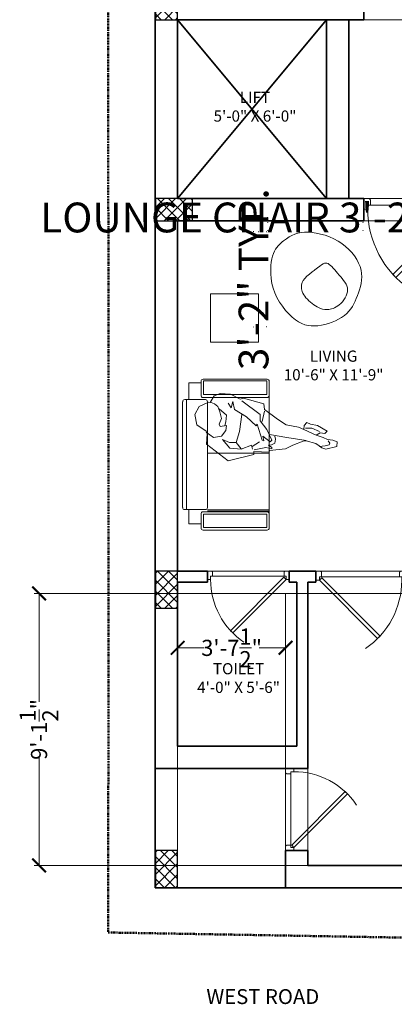
# Model space of a CAD drawing. Units: inches. Extents: x -16911 to -9621, y -48626 to -46270.
# Tile 11 of 20: x -12116 to -11965, y -46992 to -46595. Entities that reach past the tile are written whole.
import ezdxf

# ---------------------------------------------------------------- set-up
doc = ezdxf.new("R2010")
doc.units = ezdxf.units.IN
for name, pattern in [('DASHDOT', [1, 0.5, -0.25, 0, -0.25]), ('DASHED', [19.05, 12.7, -6.35]), ('DOT2', [3.175, 0, -3.175])]:
    doc.linetypes.add(name, pattern=pattern)
for name, color, linetype, lineweight in [('A-ANNO-DIMS', 2, 'Continuous', 13), ('A-ANNO-TEXT', 7, 'Continuous', 18), ('A-AREA-IDEN', 3, 'Continuous', 18), ('A-DOOR', 4, 'Continuous', 18), ('A-FURN', 8, 'Continuous', 13), ('A-WALL', 7, 'Continuous', 35), ('C-PROP', 6, 'DASHDOT', 50), ('column', 12, 'Continuous', 30), ('DOOR', 143, 'Continuous', 9), ('EXT BEAM', 132, 'Continuous', 13), ('furniture', 35, 'Continuous', 15), ('Man', 8, 'Continuous', 5), ('S-BEAM', 132, 'Continuous', 25), ('S-COLS', 1, 'Continuous', 30)]:
    doc.layers.add(name, color=color, linetype=linetype, lineweight=lineweight)
doc.styles.add('style3', font='times.ttf')
doc.styles.add('style9', font='swisscl.ttf', dxfattribs={"height": 12})
doc.dimstyles.new('Dim9', dxfattribs={"dimtxt": 10, "dimasz": 0.199219, "dimexe": 1, "dimexo": 0.5, "dimgap": 1, "dimtad": 0, "dimdec": 1, "dimzin": 0, "dimdsep": 46, "dimlunit": 4, "dimtxsty": 'style9', "dimblk": 'ARCHTICK', "dimcen": 0.09, "dimclrd": 256, "dimclrt": 256, "dimadec": 0, "dimazin": 0, "dimtfac": 1, "dimtdec": 1, "dimtix": 1, "dimtofl": 0, "dimtmove": 1, "dimatfit": 3, "dimfxl": 9, "dimtolj": 1, "dimtzin": 0, "dimlwd": -1, "dimarcsym": 0})
doc.dimstyles.new('S.S.S', dxfattribs={"dimtxt": 6.5, "dimasz": 5.5, "dimexe": 2, "dimexo": 0, "dimgap": 0.09, "dimtad": 0, "dimdec": 1, "dimzin": 3, "dimdsep": 46, "dimlunit": 4, "dimtxsty": 'style3', "dimblk": 'ARCHTICK', "dimcen": 2.5, "dimclrd": 252, "dimclre": 256, "dimclrt": 7, "dimadec": 0, "dimazin": 0, "dimtfac": 1, "dimtdec": 1, "dimtix": 1, "dimtofl": 0, "dimtmove": 0, "dimatfit": 3, "dimfxl": 2, "dimtolj": 1, "dimtzin": 0, "dimlwd": 13, "dimlwe": 15, "dimarcsym": 0})

# ---------------------------------------------------------------- blocks, each defined once
blk = doc.blocks.new('Bipman02')
blk.add_lwpolyline([(0.5871, -0.067), (0.6175, -0.0496), (0.6523, -0.0539), (0.6697, -0.0376), (0.5958, 0.0069), (0.5437, 0.0156), (0.5164, 0.0297), (0.4959, 0.0069), (0.4915, -0.0235), (0.4524, -0.0061), (0.3568, 0.0113), (0.2917, 0.0548), (0.1917, 0.1287), (0.1874, 0.1722), (0.031, 0.2156), (0.0049, 0.2069), (-0.0689, 0.2461), (-0.1471, 0.2504), (-0.1949, 0.233), (-0.2253, 0.1808), (-0.2384, 0.1852), (-0.3079, 0.1504), (-0.3426, 0.0895), (-0.3253, 0.0113), (-0.2558, -0.0365), (-0.2471, -0.0583), (-0.2514, -0.1365), (-0.0863, -0.2626), (0.1092, -0.2148), (0.1092, -0.193), (0.2265, -0.1974), (0.2308, -0.1844), (0.3525, -0.1713), (0.409, -0.1452), (0.4872, -0.1148), (0.5089, -0.1104), (0.5828, -0.1322), (0.6088, -0.1496), (0.6295, -0.1636), (0.661, -0.1757), (0.7435, -0.1539), (0.7478, -0.1191), (0.7143, -0.1051), (0.674, -0.1017), (0.6392, -0.0844)], close=True)
for points in [[(-0.2558, -0.0452), (-0.1993, -0.0844), (-0.1385, -0.0757), (-0.1037, -0.0322), (-0.0994, 0.0069), (-0.1471, -0.0018), (-0.1558, 0.0156), (-0.1385, 0.0591), (-0.1515, 0.1113), (-0.1645, 0.1504), (-0.1906, 0.1722), (-0.2167, 0.1808)], [(-0.0863, 0.1765), (-0.0646, 0.1417), (-0.0516, 0.1895), (-0.0385, 0.1287), (0.0527, 0.0722), (0.1266, 0.0026), (0.1353, 0.0156), (0.1744, -0.1061), (0.1874, -0.1104), (0.1787, -0.0757), (0.2352, -0.1191), (0.2482, -0.1061), (0.2091, -0.0235), (0.157, 0.0417), (0.157, 0.0895), (0.018, 0.1939)], [(-0.1558, 0.133), (-0.0994, 0.0852), (-0.1037, 0.033), (-0.1124, 0.0069)], [(0.018, 0.0895), (0.0006, -0.0409), (-0.0255, -0.1235), (-0.0776, -0.1235), (-0.1298, -0.1017), (-0.0733, -0.167), (0.0136, -0.1757), (0.0918, -0.1452), (0.1005, -0.1757)], [(0.1917, 0.1156), (0.1744, 0.0374)], [(0.2308, -0.0626), (0.3612, -0.0844), (0.5089, -0.1095)], [(0.4915, -0.0235), (0.5871, -0.067)], [(0.5045, -0.0148), (0.5523, -0.0148), (0.6132, -0.0409)], [(-0.0255, -0.1235), (0.0136, -0.1713)], [(0.0962, -0.1539), (0.1526, -0.1191)], [(0.2699, -0.0757), (0.2743, -0.0974), (0.2699, -0.1278), (0.2439, -0.1409), (0.2222, -0.1452), (0.2482, -0.1626), (0.2482, -0.1713), (0.2004, -0.1626), (0.1135, -0.18)], [(0.6783, -0.1104), (0.6914, -0.1278), (0.687, -0.1409), (0.6566, -0.1496), (0.6088, -0.1539)]]:
    blk.add_lwpolyline(points)
blk = doc.blocks.new('erertety')
at = {"layer": 'furniture', "ltscale": 0.2}
for p, q in [((-17662.13, -45230.66), (-17662.13, -45176.69)), ((-17693.83, -45223.2), (-17693.83, -45184.43)), ((-17685.49, -45183.68), (-17693.08, -45183.68)), ((-17684.74, -45223.2), (-17684.74, -45184.43)), ((-17684.74, -45203.31), (-17662.13, -45203.31)), ((-17685.49, -45223.95), (-17693.08, -45223.95)), ((-17691.58, -45223.95), (-17691.58, -45229.1)), ((-17684.74, -45223.99), (-17662.13, -45223.99)), ((-17684.74, -45224.55), (-17662.13, -45224.55)), ((-17684.74, -45224.55), (-17662.13, -45224.55)), ((-17691.58, -45229.1), (-17687.09, -45229.1))]:
    blk.add_line(p, q, dxfattribs=at)
blk.add_lwpolyline([(-17687.09, -45177.54), (-17691.58, -45177.54), (-17691.58, -45183.68)], dxfattribs=at)
for points in [[(-17662.13, -45182.17), (-17662.13, -45176.97, 0.414214), (-17662.87, -45176.22), (-17686.34, -45176.22, 0.414214), (-17687.09, -45176.97), (-17687.09, -45182.17, 0.414214), (-17686.34, -45182.91), (-17662.87, -45182.91, 0.414214)], [(-17662.13, -45225.47), (-17662.13, -45230.66, -0.414214), (-17662.87, -45231.41), (-17686.34, -45231.41, -0.414214), (-17687.09, -45230.66), (-17687.09, -45225.47, -0.414214), (-17686.34, -45224.72), (-17662.87, -45224.72, -0.414214)]]:
    blk.add_lwpolyline(points, format="xyb", close=True, dxfattribs=at)
for points in [[(-17663.01, -45181.75), (-17663.01, -45176.82), (-17686.21, -45176.82), (-17686.21, -45181.75)], [(-17692.4, -45183.68), (-17692.4, -45223.95), (-17692.4, -45223.95), (-17692.4, -45183.68)], [(-17663.01, -45225.6), (-17663.01, -45230.53), (-17686.21, -45230.53), (-17686.21, -45225.6)]]:
    blk.add_lwpolyline(points, close=True, dxfattribs=at)
for centre, start, end in [((-17693.08, -45184.43), 90, 180), ((-17685.49, -45184.43), 0, 90), ((-17693.08, -45223.2), 180, 270), ((-17685.49, -45223.2), 270, 0)]:
    blk.add_arc(centre, 0.748, start, end, dxfattribs=at)
at = {"layer": 'furniture', "ltscale": 0.2, "xscale": 47.90818138957024, "yscale": 47.90818138957024, "zscale": 47.90818138957024}
blk.add_blockref('Bipman02', (-17673, -45193.44, 0), dxfattribs=at)
blk = doc.blocks.new('rthrty')
at = {"layer": 'furniture'}
blk.add_open_spline([(-17650.3, -45154.53), (-17651.97, -45142.9), (-17645.3, -45136.31), (-17637.11, -45132.37), (-17620.71, -45137.17), (-17612.47, -45149.45), (-17615.73, -45159.71), (-17619.67, -45168.02), (-17632.28, -45172.65), (-17641.84, -45170.43), (-17649.5, -45159.42), (-17650.3, -45154.53)], degree=3, dxfattribs=at)
at = {"layer": 'Man'}
blk.add_open_spline([(-17632.99, -45149.02), (-17629.89, -45146.6), (-17628, -45145.12), (-17623.29, -45151.15), (-17618.06, -45156.77), (-17623.15, -45164.08), (-17628.28, -45165.32), (-17631.61, -45164.6), (-17638.01, -45159.61), (-17638.81, -45154.69), (-17636.9, -45151.81), (-17632.99, -45149.02), (-17632.99, -45149.02)], degree=3, dxfattribs=at)
blk = doc.blocks.new('A$C1C9D3E54')
at = {"layer": 'DOOR'}
blk.add_line((18676.53, 5780.72), (18710.53, 5780.72), dxfattribs=at)
blk.add_lwpolyline([(18685.01, 5806.62), (18710.47, 5781.16), (18711.53, 5782.22), (18686.07, 5807.68), (18685.01, 5806.62)], dxfattribs=at)
blk.add_lwpolyline([(18674.03, 5778.22), (18676.03, 5778.22), (18674.03, 5778.22), (18674.03, 5782.22), (18675.53, 5782.22), (18675.53, 5780.72), (18676.53, 5780.72), (18676.53, 5778.72), (18676.41, 5778.72), (18676.41, 5778.6, -0.414214), (18676.16, 5778.35), (18676.03, 5778.35), (18676.03, 5778.22)], format="xyb", dxfattribs=at)
blk.add_lwpolyline([(18713.03, 5782.22), (18711.53, 5782.22), (18711.53, 5780.72), (18710.53, 5780.72), (18710.53, 5778.72), (18710.66, 5778.72), (18710.66, 5778.6, 0.414214), (18710.91, 5778.35), (18711.03, 5778.35), (18711.03, 5778.22), (18713.03, 5778.22), (18711.03, 5778.22), (18713.03, 5778.22), (18713.03, 5782.22)], format="xyb", close=True, dxfattribs=at)
blk.add_arc((18711.53, 5782.22), 36, 124.0336, 180, dxfattribs=at)
blk = doc.blocks.new('COLUMNS')
at = {"layer": 'column'}
h = blk.add_hatch(dxfattribs=at)
h.set_pattern_fill('ANSI37', color=256, angle=-900)
h.set_pattern_definition([(225, (-45817.4075, 11499.4594), (2.24506403, -2.24506403), []), (315, (-45817.4075, 11499.4594), (2.24506403, 2.24506403), [])])
h.paths.add_polyline_path([(-12052.47, -46580.36), (-12061.47, -46580.36), (-12061.47, -46595.36), (-12052.47, -46595.36)])
h = blk.add_hatch(dxfattribs=at)
h.set_pattern_fill('ANSI37', color=256, angle=-810)
h.set_pattern_definition([(315, (-70141.2892, -80432.2886), (2.24506403, 2.24506403), []), (45, (-70141.2892, -80432.2886), (-2.24506403, 2.24506403), [])])
h.paths.add_polyline_path([(-12061.47, -46667.36), (-12061.47, -46676.36), (-12046.47, -46676.36), (-12046.47, -46667.36)])
h = blk.add_hatch(dxfattribs=at)
h.set_pattern_fill('ANSI37', color=256, angle=-540)
h.set_pattern_definition([(225, (-45817.4075, 11262.5055), (2.24506403, -2.24506403), []), (315, (-45817.4075, 11262.5055), (2.24506403, 2.24506403), [])])
h.paths.add_polyline_path([(-12052.47, -46817.31), (-12061.47, -46817.31), (-12061.47, -46832.31), (-12052.47, -46832.31)])
h = blk.add_hatch(dxfattribs=at)
h.set_pattern_fill('ANSI37', color=256, angle=-720)
h.set_pattern_definition([(45, (21703.4588, -105024.6242), (-2.24506403, 2.24506403), []), (135, (21703.4588, -105024.6242), (-2.24506403, -2.24506403), [])])
h.paths.add_polyline_path([(-12061.47, -46944.81), (-12052.47, -46944.81), (-12052.47, -46929.81), (-12061.47, -46929.81)])
at = {"layer": 'column', "ltscale": 0.05}
for points in [[(-12061.47, -46595.36), (-12052.47, -46595.36), (-12052.47, -46580.36), (-12061.47, -46580.36)], [(-12046.47, -46676.36), (-12046.47, -46667.36), (-12061.47, -46667.36), (-12061.47, -46676.36)], [(-12061.47, -46832.31), (-12052.47, -46832.31), (-12052.47, -46817.31), (-12061.47, -46817.31)], [(-12052.47, -46929.81), (-12061.47, -46929.81), (-12061.47, -46944.81), (-12052.47, -46944.81)]]:
    blk.add_lwpolyline(points, close=True, dxfattribs=at)
blk = doc.blocks.new('TYPICAL BEAMS G-2')
at = {"layer": 'EXT BEAM'}
for p, q in [((-12061.47, -48216.7), (-12061.47, -47658.74)), ((-12052.47, -47939.24), (-12052.47, -47667.74)), ((-12052.47, -47867.24), (-11924.72, -47867.24)), ((-11992.47, -47867.24), (-11992.47, -47939.24)), ((-11983.47, -47867.24), (-11983.47, -47939.24)), ((-12046.47, -47939.24), (-11929.47, -47939.24)), ((-12052.47, -48089.2), (-12052.47, -47948.24)), ((-12046.47, -47948.24), (-11929.47, -47948.24)), ((-12052.47, -48089.2), (-11747.92, -48089.2)), ((-12052.47, -48216.7), (-12052.47, -48098.2)), ((-12052.47, -48098.2), (-11879.72, -48098.2)), ((-12008.97, -48098.2), (-12008.97, -48207.7)), ((-11999.97, -48098.2), (-11999.97, -48207.7)), ((-12052.47, -48207.7), (-11879.72, -48207.7)), ((-12061.47, -48216.7), (-11738.92, -48216.7))]:
    blk.add_line(p, q, dxfattribs=at)
blk = doc.blocks.new('_ArchTick')
at = {"color": 0, "linetype": 'ByBlock', "const_width": 0.15}
blk.add_lwpolyline([(-0.5, -0.5), (0.5, 0.5)], dxfattribs=at)
blk = doc.blocks.new('*D42')
at = {"layer": 'A-ANNO-DIMS', "color": 0, "lineweight": 15, "transparency": 16777216}
for p, q in [((-12052.47, -46826.31), (-12052.47, -46850.23)), ((-12008.97, -46826.31), (-12008.97, -46850.23))]:
    blk.add_line(p, q, dxfattribs=at)
at = {"layer": 'A-ANNO-DIMS', "color": 0, "lineweight": 13, "transparency": 16777216}
for p, q in [((-12052.47, -46848.23), (-12041.79, -46848.23)), ((-12008.97, -46848.23), (-12019.66, -46848.23))]:
    blk.add_line(p, q, dxfattribs=at)
at = {"layer": 'Defpoints', "color": 0, "transparency": 16777216}
for p in [(-12052.47, -46826.31), (-12008.97, -46826.31), (-12008.97, -46848.23)]:
    blk.add_point(p, dxfattribs=at)
at = {"layer": 'A-ANNO-DIMS', "color": 0, "lineweight": 13, "transparency": 16777216, "xscale": 5.5, "yscale": 5.5, "zscale": 5.5, "rotation": 180}
blk.add_blockref('_ArchTick', (-12052.47, -46848.23), dxfattribs=at)
at = {"layer": 'A-ANNO-DIMS', "color": 0, "lineweight": 13, "transparency": 16777216, "xscale": 5.5, "yscale": 5.5, "zscale": 5.5}
blk.add_blockref('_ArchTick', (-12008.97, -46848.23), dxfattribs=at)
at = {"layer": 'A-ANNO-DIMS', "color": 0, "transparency": 16777216, "insert": (-12030.72, -46848.23), "char_height": 6.5, "attachment_point": 5, "style": 'style3'}
blk.add_mtext('\\A1;3\'-7{\\H1x;\\S1/2;}"', dxfattribs=at)
blk = doc.blocks.new('*D43')
at = {"layer": 'A-ANNO-DIMS', "color": 0, "lineweight": 15, "transparency": 16777216}
for p, q in [((-12052.47, -46826.31), (-12110.37, -46826.31)), ((-12052.47, -46935.81), (-12110.37, -46935.81))]:
    blk.add_line(p, q, dxfattribs=at)
at = {"layer": 'A-ANNO-DIMS', "color": 0, "lineweight": 13, "transparency": 16777216}
for p, q in [((-12108.37, -46826.31), (-12108.37, -46869.99)), ((-12108.37, -46935.81), (-12108.37, -46892.13))]:
    blk.add_line(p, q, dxfattribs=at)
at = {"layer": 'Defpoints', "color": 0, "transparency": 16777216}
for p in [(-12052.47, -46826.31), (-12108.37, -46935.81), (-12052.47, -46935.81)]:
    blk.add_point(p, dxfattribs=at)
at = {"layer": 'A-ANNO-DIMS', "color": 0, "lineweight": 13, "transparency": 16777216, "xscale": 5.5, "yscale": 5.5, "zscale": 5.5}
for p, rotation in [((-12108.37, -46826.31), 90), ((-12108.37, -46935.81), 270)]:
    blk.add_blockref('_ArchTick', p, dxfattribs=dict(at, rotation=rotation))
at = {"layer": 'A-ANNO-DIMS', "color": 0, "transparency": 16777216, "insert": (-12108.37, -46881.06), "char_height": 6.5, "attachment_point": 5, "rotation": 90, "style": 'style3'}
blk.add_mtext('\\A1;9\'-1{\\H1x;\\S1/2;}"', dxfattribs=at)
blk = doc.blocks.new('*D75')
at = {"layer": 'A-ANNO-DIMS', "linetype": 'DASHED', "transparency": 16777216}
for p, q in [((-12016.12, -46674.98), (-12016.32, -46674.98)), ((-11977.71, -46674.98), (-11977.51, -46674.98))]:
    blk.add_line(p, q, dxfattribs=at)
at = {"layer": 'A-ANNO-DIMS', "color": 0, "linetype": 'DOT2', "lineweight": -2, "transparency": 16777216}
for p, q in [((-12016.12, -46680.24), (-12016.12, -46673.98)), ((-11977.71, -46680.24), (-11977.71, -46673.98))]:
    blk.add_line(p, q, dxfattribs=at)
at = {"layer": 'Defpoints', "color": 0, "transparency": 16777216}
for p in [(-11977.71, -46674.98), (-12016.12, -46680.74), (-11977.71, -46680.74)]:
    blk.add_point(p, dxfattribs=at)
at = {"layer": 'A-ANNO-DIMS', "transparency": 16777216, "xscale": 0.19921875, "yscale": 0.19921875, "zscale": 0.19921875}
blk.add_blockref('_ArchTick', (-12016.12, -46674.98), dxfattribs=at)
at = {"layer": 'A-ANNO-DIMS', "transparency": 16777216, "xscale": 0.19921875, "yscale": 0.19921875, "zscale": 0.19921875, "rotation": 180}
blk.add_blockref('_ArchTick', (-11977.71, -46674.98), dxfattribs=at)
at = {"layer": 'A-ANNO-DIMS', "transparency": 16777216, "insert": (-11996.91, -46674.98), "char_height": 12, "attachment_point": 5, "style": 'style9'}
blk.add_mtext('\\A1;LOUNGE CHAIR 3\'-2 1/2" TYP.', dxfattribs=at)
blk = doc.blocks.new('*D76')
at = {"layer": 'A-ANNO-DIMS', "color": 0, "linetype": 'DOT2', "lineweight": -2, "transparency": 16777216}
for p, q in [((-12016.62, -46680.74), (-12022.88, -46680.74)), ((-12016.62, -46718.96), (-12022.88, -46718.96))]:
    blk.add_line(p, q, dxfattribs=at)
at = {"layer": 'A-ANNO-DIMS', "linetype": 'DASHED', "transparency": 16777216}
for p, q in [((-12021.88, -46680.74), (-12021.88, -46680.54)), ((-12021.88, -46718.96), (-12021.88, -46719.16))]:
    blk.add_line(p, q, dxfattribs=at)
at = {"layer": 'Defpoints', "color": 0, "transparency": 16777216}
for p in [(-12021.88, -46680.74), (-12016.12, -46680.74), (-12016.12, -46718.96)]:
    blk.add_point(p, dxfattribs=at)
at = {"layer": 'A-ANNO-DIMS', "transparency": 16777216, "xscale": 0.19921875, "yscale": 0.19921875, "zscale": 0.19921875}
for p, rotation in [((-12021.88, -46680.74), 270), ((-12021.88, -46718.96), 90)]:
    blk.add_blockref('_ArchTick', p, dxfattribs=dict(at, rotation=rotation))
at = {"layer": 'A-ANNO-DIMS', "transparency": 16777216, "insert": (-12021.88, -46699.85), "char_height": 12, "attachment_point": 5, "rotation": 90, "style": 'style9'}
blk.add_mtext('\\A1;3\'-2" TYP.', dxfattribs=at)

msp = doc.modelspace()

# ---------------------------------------------------------------- linework, layer by layer
at = {"layer": 'A-FURN'}
msp.add_lwpolyline([(-12019.878, -46705.751), (-12039.238, -46705.751), (-12039.238, -46725.111), (-12019.878, -46725.111)], close=True, dxfattribs=at)
at = {"layer": 'A-WALL'}
for p, q in [((-12061.474, -46896.809), (-12061.474, -46434.855)), ((-11977.474, -46595.355), (-11977.474, -46586.355)), ((-12052.474, -46667.355), (-12052.474, -46595.355)), ((-11977.474, -46595.355), (-12052.474, -46595.355)), ((-12052.474, -46595.355), (-11992.474, -46667.355)), ((-12052.474, -46667.355), (-11992.474, -46595.355)), ((-11992.474, -46667.355), (-11992.474, -46595.355)), ((-11983.474, -46667.355), (-11983.474, -46595.355)), ((-11977.474, -46667.355), (-12052.474, -46667.355)), ((-11977.474, -46676.355), (-11977.474, -46667.355)), ((-12052.474, -46817.309), (-12052.474, -46676.355)), ((-11977.474, -46676.355), (-12052.474, -46676.355)), ((-12052.474, -46817.309), (-12040.474, -46817.309)), ((-12040.474, -46817.309), (-12040.474, -46821.809)), ((-12007.474, -46817.309), (-11996.724, -46817.309)), ((-12007.474, -46817.309), (-12007.474, -46821.809)), ((-11996.724, -46821.809), (-11996.724, -46817.309)), ((-12052.474, -46887.809), (-12052.474, -46821.809)), ((-12052.474, -46821.809), (-12040.474, -46821.809)), ((-12007.474, -46821.809), (-12004.474, -46821.809)), ((-12004.474, -46887.809), (-12004.474, -46821.809)), ((-11999.974, -46896.809), (-11999.974, -46821.809)), ((-11999.974, -46821.809), (-11996.724, -46821.809)), ((-12052.474, -46887.809), (-12004.474, -46887.809)), ((-12061.474, -46944.809), (-12061.474, -46896.809)), ((-12061.474, -46896.809), (-11999.974, -46896.809)), ((-12008.974, -46944.809), (-12008.974, -46929.809)), ((-12008.974, -46929.809), (-11999.974, -46929.809)), ((-11999.974, -46935.809), (-11999.974, -46929.809)), ((-11999.974, -46935.809), (-11879.724, -46935.809)), ((-12061.474, -46944.809), (-12008.974, -46944.809)), ((-12008.974, -46944.809), (-11738.925, -46944.809))]:
    msp.add_line(p, q, dxfattribs=at)
at = {"layer": 'C-PROP'}
msp.add_lwpolyline([(-12080.474, -46962.809), (-11720.293, -46969.035), (-11719.732, -46940.446), (-11720.395, -46855.606), (-11721.561, -46609.511), (-11721.175, -46367.855), (-12080.838, -46362.811), (-12080.3, -46762.955)], close=True, dxfattribs=at)

# ---------------------------------------------------------------- block references
at = {"layer": 'A-DOOR'}
for p, xscale, yscale, zscale, rotation in [((-32087.969, -40444.653), -1.076923076922859, 1.076923076922859, 1.076923076922859, 180), ((-27841.577, -41928.043), -0.8461538461538624, 0.8461538461538624, 0.8461538461538624, 180), ((5276.842, -41483.564), 0.9230769230769229, 0.9230769230769229, 0.9230769230769229, 180), ((-16898.241, -31095.706), 0.8461538461538624, 0.8461538461538624, 0.8461538461538624, 270)]:
    msp.add_blockref('A$C1C9D3E54', p, dxfattribs=dict(at, xscale=xscale, yscale=yscale, zscale=zscale, rotation=rotation))
at = {"layer": 'A-FURN'}
msp.add_blockref('rthrty', (5635.852, -1547.053), dxfattribs=at)
at = {"layer": 'A-FURN', "xscale": 1.1, "yscale": 1.1, "zscale": 1.1}
msp.add_blockref('erertety', (7412.76, 2953.75, 0), dxfattribs=at)
at = {"layer": 'S-BEAM'}
msp.add_blockref('TYPICAL BEAMS G-2', (0, 1271.886), dxfattribs=at)
at = {"layer": 'S-COLS'}
msp.add_blockref('COLUMNS', (0, 0), dxfattribs=at)

# ---------------------------------------------------------------- texts
at = {"layer": 'A-ANNO-TEXT', "ltscale": 10, "insert": (-12040.885, -46985.611), "char_height": 6, "width": 70.69764, "attachment_point": 1, "style": 'style9'}
msp.add_mtext('\\A1;{\\fCentury Gothic|b0|i0|c0|p34;WEST ROAD}', dxfattribs=at)
at = {"layer": 'A-AREA-IDEN', "ltscale": 10, "char_height": 4.5, "width": 42.823, "attachment_point": 1, "style": 'style9'}
for s, insert in [('\\A1;\\pxqc;{\\fCentury Gothic|b0|i0|c0|p34;LIFT\\P5\'-0" X 6\'-0"}', (-12042.698, -46624.39)), ('\\A1;\\pxqc;{\\fCentury Gothic|b0|i0|c0|p34;LIVING\\P10\'-6" X 11\'-9"}', (-12011.012, -46728.541)), ('\\A1;\\pxqc;{\\fCentury Gothic|b0|i0|c0|p34;TOILET\\P4\'-0" X 5\'-6"}', (-12049.33, -46854.373))]:
    msp.add_mtext(s, dxfattribs=dict(at, insert=insert))

# ---------------------------------------------------------------- dimensions: what is measured, and where the dimension line sits
at = {"layer": 'A-ANNO-DIMS'}
dim = msp.add_linear_dim(base=(-11977.706, -46674.975), p1=(-12016.121, -46680.738), p2=(-11977.706, -46680.738), text='LOUNGE CHAIR <> TYP.', dimstyle='Dim9', override={"dimdec": 1, "dimrnd": 0, "dimzin": 1, "dimlunit": 4, "dimfrac": 2}, dxfattribs=at)
dim.commit()
dim.dimension.update_dxf_attribs({"geometry": '*D75', "text_midpoint": (-11996.914, -46674.975)})
dim = msp.add_linear_dim(base=(-12021.883, -46680.738), p1=(-12016.121, -46718.962), p2=(-12016.121, -46680.738), angle=90, text='<> TYP.', dimstyle='Dim9', override={"dimdec": 1, "dimrnd": 0, "dimzin": 1, "dimlunit": 4, "dimfrac": 2}, dxfattribs=at)
dim.commit()
dim.dimension.update_dxf_attribs({"geometry": '*D76', "text_midpoint": (-12021.883, -46699.85)})
dim = msp.add_linear_dim(base=(-12108.373, -46935.809), p1=(-12052.474, -46826.309), p2=(-12052.474, -46935.809), angle=90, dimstyle='S.S.S', override={"dimclrd": 0, "dimclre": 0, "dimclrt": 0}, dxfattribs=at)
dim.commit()
dim.dimension.update_dxf_attribs({"geometry": '*D43', "text_midpoint": (-12108.373, -46881.059)})
dim = msp.add_linear_dim(base=(-12008.974, -46848.227), p1=(-12052.474, -46826.309), p2=(-12008.974, -46826.309), dimstyle='S.S.S', override={"dimclrd": 0, "dimclre": 0, "dimclrt": 0}, dxfattribs=at)
dim.commit()
dim.dimension.update_dxf_attribs({"geometry": '*D42', "text_midpoint": (-12030.724, -46848.227)})

doc.saveas('drawing.dxf')
